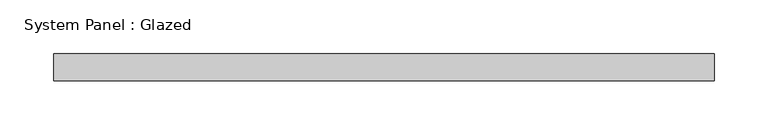
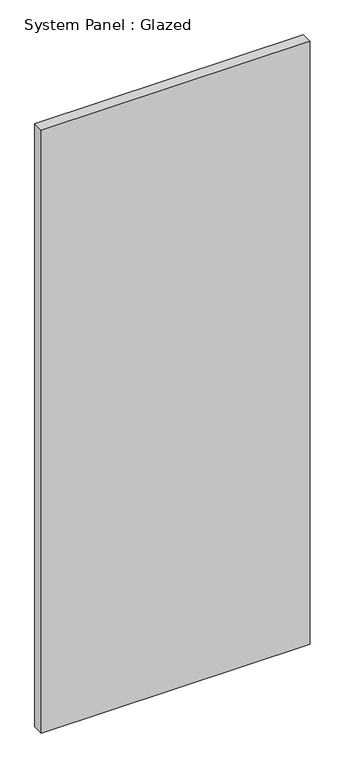
"""IFC4 building model written with IfcOpenShell, lengths in millimetres: plate geometry, System Panel : Glazed."""

from ifc_helpers import new_model, si_unit, origin, origin_with_axes, place, context, project, spatial, polyline, outline, extrude, source, transform, mapped, element, save


def system_panel_glazed_fad1f0ba(model_context):
    return source(origin(), model_context, "Body", "SweptSolid", [
        extrude(outline(polyline([(307.975, 19.05), (-307.975, 19.05), (-307.975, 44.45), (307.975, 44.45), (307.975, 19.05)])), origin_with_axes(), (0.0, 0.0, 1.0), 1459.2856263),
    ])


if __name__ == "__main__":
    model = new_model("IFC4")
    model_context = context("Model", 3, world=origin())
    ifc_project = project(units=[si_unit("LENGTHUNIT", "METRE", prefix="MILLI")], contexts=[model_context])
    site = spatial("IfcSite", under=ifc_project)
    building = spatial("IfcBuilding", under=site)
    placement = place(None, origin())
    system_panel_glazed_shape = system_panel_glazed_fad1f0ba(model_context)
    element("IfcPlate", 1, ObjectType="System Panel : Glazed", at=placement, inside=building, context=model_context, shape_type="MappedRepresentation", body=[
        mapped(system_panel_glazed_shape, transform((0.0, 0.0, 0.0), x_axis=(1.0, 0.0, 0.0), y_axis=(0.0, 1.0, 0.0), z_axis=(0.0, 0.0, 1.0))),
    ])
    save(model, "model.ifc")

# Revit data of these elements
# Type "System Panel : Glazed"
#   Construction Type Id = "GSP4R"
#   Analytic Construction = "1/8 in Pilkington single glazing"
#   Visual Light Transmittance = 0.9
#   Solar Heat Gain Coefficient = 0.86
#   Heat Transfer Coefficient (U) = 1.18115 BTU/(h·ft²·°F)
#   Define Thermal Properties by = 1
# Element 1 (IfcPlate, "System Panel : Glazed")
#   Materials on its faces: "Glass"
# Materials
#   "Glass": class "Glass", colour RGB 0 128 192, transparency 0.75, Description = "Soda Lime Glass", Cost = 0
